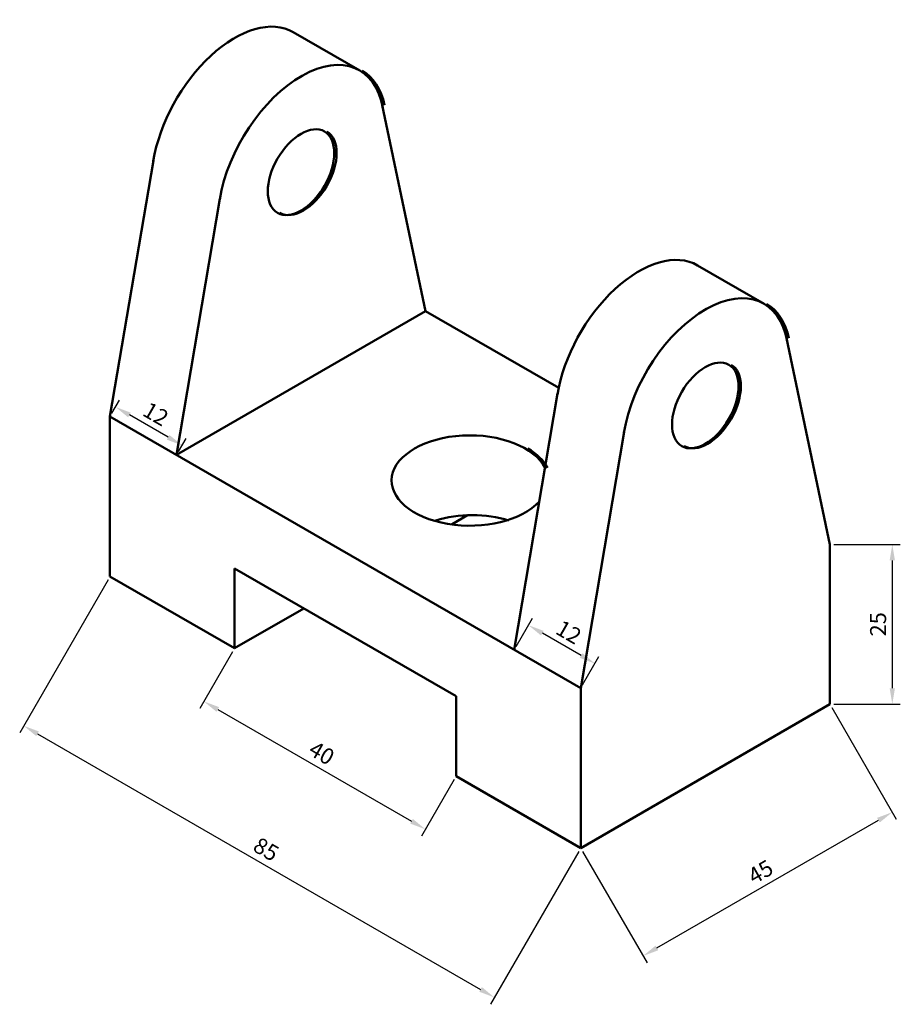
# Model space of a CAD drawing. Units: millimetres. Extents: x 83532273 to 83532410, y 29006806 to 29006960.
import ezdxf

# ---------------------------------------------------------------- set-up
doc = ezdxf.new("R2010")
doc.units = ezdxf.units.MM
doc.layers.add('M-DIMS', color=2, linetype='Continuous', lineweight=25)
doc.layers.add('M-OUTL', color=7, linetype='Continuous', lineweight=50)
doc.styles.get("Standard").update_dxf_attribs({"font": 'arial.ttf'})
doc.dimstyles.new('ISO-25', dxfattribs={"dimtxt": 2.5, "dimasz": 2.5, "dimexe": 1.25, "dimexo": 0.625, "dimtad": 1, "dimtxsty": 'Standard', "dimcen": 2.5, "dimadec": 0, "dimazin": 0, "dimtfac": 1, "dimtmove": 0, "dimatfit": 3, "dimfxl": 1, "dimarcsym": 0})

# ---------------------------------------------------------------- blocks, each defined once
blk = doc.blocks.new('*D1')
at = {"layer": 'Defpoints', "color": 0, "transparency": 16777216}
for p in [(83532306.3, 29006861.82), (83532340.94, 29006841.82), (83532336.14, 29006833.5)]:
    blk.add_point(p, dxfattribs=at)
at = {"layer": 'M-DIMS', "color": 0, "lineweight": -2, "transparency": 16777216}
for p, q in [((83532305.99, 29006861.28), (83532300.88, 29006852.42)), ((83532303.67, 29006852.25), (83532333.98, 29006834.75)), ((83532340.63, 29006841.28), (83532335.52, 29006832.42))]:
    blk.add_line(p, q, dxfattribs=at)
at = {"layer": 'M-DIMS', "color": 0, "transparency": 16777216}
for points in [[(83532303.88, 29006852.61), (83532303.46, 29006851.89), (83532301.5, 29006853.5)], [(83532334.19, 29006835.11), (83532333.77, 29006834.39), (83532336.14, 29006833.5)]]:
    blk.add_solid(points, dxfattribs=at)
at = {"layer": 'M-DIMS', "color": 0, "transparency": 16777216, "insert": (83532319.77, 29006845.15), "char_height": 2.5, "attachment_point": 5, "rotation": 330}
blk.add_mtext('40', dxfattribs=at)
blk = doc.blocks.new('*D2')
at = {"layer": 'Defpoints', "color": 0, "transparency": 16777216}
for p in [(83532286.82, 29006873.07), (83532360.43, 29006830.57), (83532346.93, 29006807.19)]:
    blk.add_point(p, dxfattribs=at)
at = {"layer": 'M-DIMS', "color": 0, "lineweight": -2, "transparency": 16777216}
for p, q in [((83532286.51, 29006872.53), (83532272.7, 29006848.61)), ((83532275.49, 29006848.44), (83532344.77, 29006808.44)), ((83532360.12, 29006830.03), (83532346.31, 29006806.11))]:
    blk.add_line(p, q, dxfattribs=at)
at = {"layer": 'M-DIMS', "color": 0, "transparency": 16777216}
for points in [[(83532275.7, 29006848.8), (83532275.28, 29006848.08), (83532273.32, 29006849.69)], [(83532344.98, 29006808.8), (83532344.56, 29006808.08), (83532346.93, 29006807.19)]]:
    blk.add_solid(points, dxfattribs=at)
at = {"layer": 'M-DIMS', "color": 0, "transparency": 16777216, "insert": (83532311.08, 29006830.09), "char_height": 2.5, "attachment_point": 5, "rotation": 330}
blk.add_mtext('85', dxfattribs=at)
blk = doc.blocks.new('*D3')
at = {"layer": 'Defpoints', "color": 0, "transparency": 16777216}
for p in [(83532399.4, 29006853.07), (83532409.16, 29006836.17), (83532360.43, 29006830.57)]:
    blk.add_point(p, dxfattribs=at)
at = {"layer": 'M-DIMS', "color": 0, "lineweight": -2, "transparency": 16777216}
for p, q in [((83532399.71, 29006852.53), (83532409.78, 29006835.09)), ((83532372.35, 29006814.92), (83532406.99, 29006834.92)), ((83532360.74, 29006830.03), (83532370.81, 29006812.59))]:
    blk.add_line(p, q, dxfattribs=at)
at = {"layer": 'M-DIMS', "color": 0, "transparency": 16777216}
for points in [[(83532406.78, 29006835.28), (83532407.2, 29006834.56), (83532409.16, 29006836.17)], [(83532372.14, 29006815.28), (83532372.56, 29006814.56), (83532370.18, 29006813.67)]]:
    blk.add_solid(points, dxfattribs=at)
at = {"layer": 'M-DIMS', "color": 0, "transparency": 16777216, "insert": (83532388.72, 29006826.56), "char_height": 2.5, "attachment_point": 5, "rotation": 30}
blk.add_mtext('45', dxfattribs=at)
blk = doc.blocks.new('*D4')
at = {"layer": 'Defpoints', "color": 0, "transparency": 16777216}
for p in [(83532399.4, 29006878.07), (83532399.4, 29006853.07), (83532409.17, 29006853.07)]:
    blk.add_point(p, dxfattribs=at)
at = {"layer": 'M-DIMS', "color": 0, "lineweight": -2, "transparency": 16777216}
for p, q in [((83532400.03, 29006878.07), (83532410.42, 29006878.07)), ((83532409.17, 29006875.57), (83532409.17, 29006855.57)), ((83532400.03, 29006853.07), (83532410.42, 29006853.07))]:
    blk.add_line(p, q, dxfattribs=at)
at = {"layer": 'M-DIMS', "color": 0, "transparency": 16777216}
for points in [[(83532408.75, 29006875.57), (83532409.58, 29006875.57), (83532409.17, 29006878.07)], [(83532408.75, 29006855.57), (83532409.58, 29006855.57), (83532409.17, 29006853.07)]]:
    blk.add_solid(points, dxfattribs=at)
at = {"layer": 'M-DIMS', "color": 0, "transparency": 16777216, "insert": (83532407.27, 29006865.57), "char_height": 2.5, "attachment_point": 5, "rotation": 90}
blk.add_mtext('25', dxfattribs=at)
blk = doc.blocks.new('*D5')
at = {"layer": 'Defpoints', "color": 0, "transparency": 16777216}
for p in [(83532352.27, 29006865.43), (83532350.04, 29006861.57), (83532360.43, 29006855.57)]:
    blk.add_point(p, dxfattribs=at)
at = {"layer": 'M-DIMS', "color": 0, "lineweight": -2, "transparency": 16777216}
for p, q in [((83532350.35, 29006862.11), (83532352.9, 29006866.52)), ((83532360.5, 29006860.68), (83532354.44, 29006864.18)), ((83532360.74, 29006856.11), (83532363.29, 29006860.52))]:
    blk.add_line(p, q, dxfattribs=at)
at = {"layer": 'M-DIMS', "color": 0, "transparency": 16777216}
for points in [[(83532354.64, 29006864.54), (83532354.23, 29006863.82), (83532352.27, 29006865.43)], [(83532360.71, 29006861.04), (83532360.29, 29006860.32), (83532362.66, 29006859.43)]]:
    blk.add_solid(points, dxfattribs=at)
at = {"layer": 'M-DIMS', "color": 0, "transparency": 16777216, "insert": (83532358.41, 29006864.06), "char_height": 2.5, "attachment_point": 5, "rotation": 330}
blk.add_mtext('12', dxfattribs=at)
blk = doc.blocks.new('*D6')
at = {"layer": 'Defpoints', "color": 0, "transparency": 16777216}
for p in [(83532287.69, 29006899.58), (83532286.82, 29006898.07), (83532297.21, 29006892.07)]:
    blk.add_point(p, dxfattribs=at)
at = {"layer": 'M-DIMS', "color": 0, "lineweight": -2, "transparency": 16777216}
for p, q in [((83532287.13, 29006898.61), (83532288.31, 29006900.66)), ((83532295.92, 29006894.83), (83532289.85, 29006898.33)), ((83532297.52, 29006892.61), (83532298.71, 29006894.66))]:
    blk.add_line(p, q, dxfattribs=at)
at = {"layer": 'M-DIMS', "color": 0, "transparency": 16777216}
for points in [[(83532290.06, 29006898.69), (83532289.65, 29006897.96), (83532287.69, 29006899.58)], [(83532296.12, 29006895.19), (83532295.71, 29006894.46), (83532298.08, 29006893.58)]]:
    blk.add_solid(points, dxfattribs=at)
at = {"layer": 'M-DIMS', "color": 0, "transparency": 16777216, "insert": (83532293.83, 29006898.2), "char_height": 2.5, "attachment_point": 5, "rotation": 330}
blk.add_mtext('12', dxfattribs=at)

msp = doc.modelspace()

# ---------------------------------------------------------------- linework, layer by layer
at = {"layer": 'M-OUTL'}
for p, q in [((83532325.882, 29006952.226), (83532315.489, 29006958.226)), ((83532315.489, 29006958.226), (83532315.489, 29006958.226)), ((83532336.182, 29006914.566), (83532329.392, 29006946.823)), ((83532286.818, 29006898.066), (83532293.608, 29006938.164)), ((83532297.211, 29006892.066), (83532304.001, 29006932.164)), ((83532389.102, 29006915.726), (83532378.709, 29006921.726)), ((83532378.709, 29006921.726), (83532378.709, 29006921.726)), ((83532297.211, 29006892.066), (83532336.182, 29006914.566)), ((83532336.182, 29006914.566), (83532356.996, 29006902.549)), ((83532399.402, 29006878.066), (83532392.612, 29006910.323)), ((83532350.038, 29006861.566), (83532356.828, 29006901.664)), ((83532360.43, 29006855.566), (83532286.818, 29006898.066)), ((83532286.818, 29006898.066), (83532286.818, 29006873.066)), ((83532360.43, 29006855.566), (83532367.22, 29006895.664)), ((83532340.311, 29006881.235), (83532342.714, 29006882.622)), ((83532399.402, 29006853.066), (83532399.402, 29006878.066)), ((83532323.624, 29006876.816), (83532323.624, 29006876.816)), ((83532306.304, 29006861.816), (83532306.304, 29006874.316)), ((83532306.304, 29006874.316), (83532340.945, 29006854.316)), ((83532286.818, 29006873.066), (83532306.304, 29006861.816)), ((83532306.304, 29006861.816), (83532317.129, 29006868.066)), ((83532340.945, 29006854.316), (83532340.945, 29006841.816)), ((83532360.43, 29006830.566), (83532360.43, 29006855.566)), ((83532360.43, 29006830.566), (83532399.402, 29006853.066)), ((83532340.945, 29006841.816), (83532360.43, 29006830.566))]:
    msp.add_line(p, q, dxfattribs=at)
for centre, major_axis, start_param, end_param in [((83532306.304, 29006942.316), (-9.186, -15.91), 3.1415566, 5.2929564), ((83532316.696, 29006936.316), (-9.186, -15.91), 2.5351546, 5.2929564), ((83532306.304, 29006942.316), (-9.186, -15.91), 2.5351546, 2.5403284), ((83532317.068, 29006936.315), (-9.186, -15.91), 2.569593, 3.1415927), ((83532317.068, 29006936.315), (3.674, 6.364), 3.1415927, 6.2831853), ((83532369.524, 29006905.816), (-9.186, -15.91), 3.1415566, 5.2929564), ((83532379.916, 29006899.816), (-9.186, -15.91), 2.5351546, 5.2929564), ((83532369.524, 29006905.816), (-9.186, -15.91), 2.5351546, 2.5403284), ((83532380.287, 29006899.815), (-9.186, -15.91), 2.569593, 3.1415927), ((83532380.287, 29006899.815), (3.674, 6.364), 3.1415927, 6.2831853), ((83532343.11, 29006888.066), (-12.247, 0), 3.4268402, 8.9446171), ((83532343.481, 29006888.065), (12.247, 0), 0.2852524, 0.7853982), ((83532343.481, 29006875.565), (12.247, 0), 1.0841014, 2.0574913)]:
    msp.add_ellipse(centre, major_axis=major_axis, ratio=0.5773503, start_param=start_param, end_param=end_param, dxfattribs=at)
for centre in [(83532316.696, 29006936.316), (83532379.916, 29006899.816)]:
    msp.add_ellipse(centre, major_axis=(-3.674, -6.364), ratio=0.5773503, dxfattribs=at)

# ---------------------------------------------------------------- dimensions: what is measured, and where the dimension line sits
at = {"layer": 'M-DIMS'}
for p1, p2, distance, picture, middle in [((83532297.211, 29006892.066), (83532286.818, 29006898.066), -1.742, '*D6', (83532293.826, 29006898.203)), ((83532399.402, 29006878.066), (83532399.402, 29006853.066), 9.766, '*D4', (83532407.266, 29006865.566)), ((83532286.818, 29006873.066), (83532360.43, 29006830.566), -26.991, '*D2', (83532311.08, 29006830.088)), ((83532360.43, 29006855.566), (83532350.038, 29006861.566), -4.465, '*D5', (83532358.407, 29006864.062)), ((83532306.304, 29006861.816), (83532340.945, 29006841.816), -9.604, '*D1', (83532319.773, 29006845.145)), ((83532360.43, 29006830.566), (83532399.402, 29006853.066), -19.507, '*D3', (83532388.722, 29006826.565))]:
    dim = msp.add_aligned_dim(p1=p1, p2=p2, distance=distance, dimstyle='ISO-25', override={"dimclrd": 0, "dimclre": 0, "dimclrt": 0}, dxfattribs=at)
    dim.commit()
    dim.dimension.update_dxf_attribs({"geometry": picture, "text_midpoint": middle})

doc.saveas('drawing.dxf')
